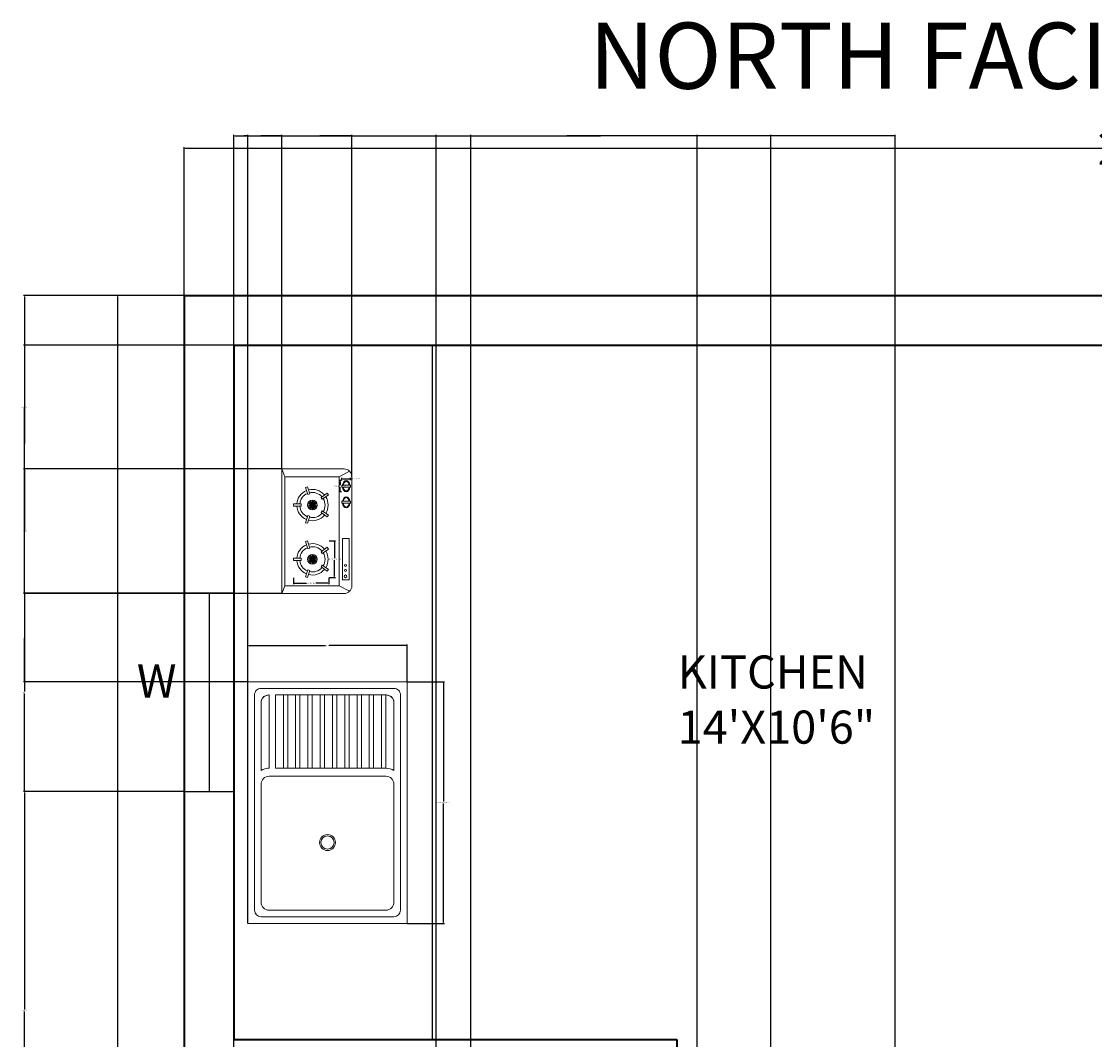
# Model space of a CAD drawing. Units: inches. Extents: x 3 to 420, y -502 to 54.
# Tile 5 of 6: x 3 to 198, y -130 to 54. Entities that reach past the tile are written whole.
import ezdxf

# ---------------------------------------------------------------- set-up
doc = ezdxf.new("R2010")
doc.units = ezdxf.units.IN
doc.header["$MEASUREMENT"] = 0
for name, color, linetype, lineweight in [('A-ANNO-DIMS', 2, 'Continuous', 18), ('A-ANNO-TEXT', 7, 'Continuous', 18), ('A-AREA-IDEN', 7, 'Continuous', 18), ('A-EQPM', 9, 'Continuous', 18), ('A-FLOR-CASE', 9, 'Continuous', 25), ('A-FLOR-FIXT', 9, 'Continuous', 18), ('A-GLAZ', 40, 'Continuous', 25), ('A-WALL', 7, 'Continuous', 35)]:
    doc.layers.add(name, color=color, linetype=linetype, lineweight=lineweight)
doc.styles.get("Standard").update_dxf_attribs({"font": 'arial.ttf'})
doc.dimstyles.get("Standard").update_dxf_attribs({"dimtxt": 0.18, "dimasz": 0.18, "dimexe": 0.18, "dimexo": 0.0625, "dimgap": 0.09, "dimtad": 0, "dimtih": 1, "dimtoh": 1, "dimdec": 0, "dimzin": 0, "dimdsep": 46, "dimlunit": 3, "dimtxsty": 'Standard', "dimcen": 0.09, "dimadec": 0, "dimazin": 0, "dimtfac": 1, "dimtdec": 0, "dimtofl": 0, "dimtmove": 0, "dimatfit": 3, "dimfxl": 1, "dimtolj": 1, "dimtzin": 0, "dimarcsym": 0})

# ---------------------------------------------------------------- blocks, each defined once
blk = doc.blocks.new('*D1')
at = {"layer": 'A-ANNO-DIMS', "color": 0, "lineweight": -2, "transparency": 16777216}
for p, q in [((32.39, 4.61), (32.39, 31.47)), ((32.57, 31.29), (198.86, 31.29)), ((390.71, 31.29), (224.42, 31.29)), ((390.89, 4.61), (390.89, 31.47))]:
    blk.add_line(p, q, dxfattribs=at)
at = {"layer": 'A-ANNO-DIMS', "color": 0, "transparency": 16777216}
for points in [[(32.57, 31.32), (32.57, 31.26), (32.39, 31.29)], [(390.71, 31.32), (390.71, 31.26), (390.89, 31.29)]]:
    blk.add_solid(points, dxfattribs=at)
at = {"layer": 'Defpoints', "color": 0, "transparency": 16777216}
for p in [(390.89, 31.29), (32.39, 4.54), (390.89, 4.54)]:
    blk.add_point(p, dxfattribs=at)
at = {"layer": 'A-ANNO-DIMS', "color": 0, "transparency": 16777216, "insert": (211.64, 31.29), "char_height": 6, "attachment_point": 5}
blk.add_mtext('\\A1;29\'-11"', dxfattribs=at)
blk = doc.blocks.new('*D2')
at = {"layer": 'A-ANNO-DIMS', "color": 0, "lineweight": -2, "transparency": 16777216}
for p, q in [((32.33, 4.54), (20.1, 4.54)), ((20.28, 4.36), (20.28, -230.8)), ((20.28, -472.28), (20.28, -237.11)), ((32.33, -472.46), (20.1, -472.46))]:
    blk.add_line(p, q, dxfattribs=at)
at = {"layer": 'A-ANNO-DIMS', "color": 0, "transparency": 16777216}
for points in [[(20.25, 4.36), (20.31, 4.36), (20.28, 4.54)], [(20.25, -472.28), (20.31, -472.28), (20.28, -472.46)]]:
    blk.add_solid(points, dxfattribs=at)
at = {"layer": 'Defpoints', "color": 0, "transparency": 16777216}
for p in [(32.39, 4.54), (20.28, -472.46), (32.39, -472.46)]:
    blk.add_point(p, dxfattribs=at)
at = {"layer": 'A-ANNO-DIMS', "color": 0, "transparency": 16777216, "insert": (20.28, -233.96), "char_height": 6, "attachment_point": 5}
blk.add_mtext('\\A1;39\'-9"', dxfattribs=at)
blk = doc.blocks.new('М12 540х820')
for p, q in [((0, 540), (-820, 540)), ((-820, 540), (-820, 0)), ((-45, 517.5), (-775, 517.5)), ((0, 0), (0, 540)), ((-797.5, 495), (-797.5, 45)), ((-347.5, 495), (-748, 495)), ((-301.7, 495), (-64.8, 495)), ((-22.5, 45), (-22.5, 495)), ((-775, 468), (-775, 72)), ((-320.5, 468), (-320.5, 72)), ((-293.7, 468), (-293.7, 472.5)), ((-293.7, 468), (-45, 468)), ((-293.7, 446.6), (-45, 446.6)), ((-293.7, 419.6), (-293.7, 446.6)), ((-45, 469.5), (-45, 468)), ((-45, 419.6), (-45, 446.6)), ((-293.7, 419.6), (-45, 419.6)), ((-293.7, 405), (-45, 405)), ((-293.7, 378), (-293.7, 405)), ((-45, 378), (-45, 405)), ((-293.7, 378), (-45, 378)), ((-293.7, 336.4), (-293.7, 363.4)), ((-293.7, 363.4), (-45, 363.4)), ((-293.7, 336.4), (-45, 336.4)), ((-45, 336.4), (-45, 363.4)), ((-293.7, 294.7), (-293.7, 321.7)), ((-293.7, 321.7), (-45, 321.7)), ((-293.7, 294.7), (-45, 294.7)), ((-45, 294.7), (-45, 321.7)), ((-293.7, 253.1), (-293.7, 280.1)), ((-293.7, 280.1), (-45, 280.1)), ((-45, 253.1), (-45, 280.1)), ((-293.7, 253.1), (-45, 253.1)), ((-293.7, 211.5), (-293.7, 238.5)), ((-293.7, 238.5), (-45, 238.5)), ((-45, 211.5), (-45, 238.5)), ((-293.7, 211.5), (-45, 211.5)), ((-293.7, 169.9), (-293.7, 196.9)), ((-293.7, 196.9), (-45, 196.9)), ((-45, 169.9), (-45, 196.9)), ((-293.7, 169.9), (-45, 169.9)), ((-293.7, 128.2), (-293.7, 155.2)), ((-293.7, 155.2), (-45, 155.2)), ((-45, 128.2), (-45, 155.2)), ((-293.7, 128.2), (-45, 128.2)), ((-293.7, 113.6), (-45, 113.6)), ((-293.7, 86.6), (-293.7, 113.6)), ((-45, 86.6), (-45, 113.6)), ((-293.7, 86.6), (-45, 86.6)), ((-748, 45), (-347.5, 45)), ((-301.7, 45), (-64.8, 45)), ((-293.7, 72), (-45, 72)), ((-45, 70.5), (-45, 72)), ((-820, 0), (0, 0)), ((-775, 22.5), (-45, 22.5))]:
    blk.add_line(p, q)
at = {"ltscale": 0.06}
for p, q in [((-820, 0), (-820, 540)), ((-820, 540), (0, 540)), ((0, 540), (0, 536.9)), ((0, 536.9), (0, 0)), ((-293.7, 446.6), (-45, 446.6)), ((-293.7, 405), (-293.7, 446.6)), ((-45, 446.6), (-45, 419.6)), ((-293.7, 363.4), (-293.7, 405)), ((-45, 419.6), (-45, 378)), ((-45, 378), (-45, 336.4)), ((-293.7, 321.7), (-293.7, 363.4)), ((-45, 336.4), (-45, 294.7)), ((-293.7, 280.1), (-293.7, 321.7)), ((-45, 294.7), (-45, 253.1)), ((-293.7, 238.5), (-293.7, 280.1)), ((-293.7, 196.9), (-293.7, 238.5)), ((-45, 253.1), (-45, 211.5)), ((-293.7, 155.2), (-293.7, 196.9)), ((-45, 211.5), (-45, 169.9)), ((-293.7, 113.6), (-293.7, 155.2)), ((-45, 169.9), (-45, 128.2)), ((-293.7, 72), (-293.7, 113.6)), ((-45, 128.2), (-45, 86.6)), ((-45, 86.6), (-45, 72)), ((-45, 72), (-293.7, 72)), ((0, 0), (-820, 0))]:
    blk.add_line(p, q, dxfattribs=at)
at = {"extrusion": (0, 0, -1)}
for centre, major_axis, start_param, end_param in [((-775, 495), (-15.9, 15.9), -0.785398, 0.785398), ((-775, 495), (-15.9, 15.9), -0.785398, 0.785398), ((-45, 495), (-15.9, -15.9), 2.356194, 3.926991), ((-45, 495), (-15.9, -15.9), 2.356194, 3.926991), ((-748, 468), (-19.1, -19.1), 0.785398, 2.356194), ((-748, 468), (-19.1, -19.1), 0.785398, 2.356194), ((-347.5, 468), (-19.1, 19.1), 0.785398, 2.356194), ((-347.5, 468), (-19.1, 19.1), 0.785398, 2.356194), ((-343.2, 468), (-35, 35), 1.779263, 2.356194), ((-343.2, 468), (-35, 35), 1.779263, 2.356192), ((-72.3, 468.8), (-19.3, 19.3), 1.0328, 2.38382), ((-72.3, 468.8), (-19.3, 19.3), 1.0328, 1.064673), ((-72.3, 468.8), (-19.3, 19.3), 1.064673, 2.328569), ((-343.2, 468), (-35, 35), 2.356192, 2.356194), ((-72.3, 468.8), (-19.3, 19.3), 2.328569, 2.38382), ((-545.5, 270), (-19.1, -19.1), 3.926991, 10.210176), ((-545.5, 270), (-19.1, -19.1), 3.926991, 10.210176), ((-545.5, 270), (-15.9, -15.9), 3.926991, 10.210176), ((-545.5, 270), (-15.9, -15.9), 3.926991, 10.210176), ((-775, 45), (-15.9, -15.9), 5.497787, 7.068583), ((-775, 45), (-15.9, -15.9), 5.497787, 7.068583), ((-748, 72), (-19.1, 19.1), 3.926991, 5.497787), ((-748, 72), (-19.1, 19.1), 3.926991, 5.497787), ((-347.5, 72), (-19.1, -19.1), 3.926991, 5.497787), ((-347.5, 72), (-19.1, -19.1), 3.926991, 5.497787), ((-343.2, 72), (-35, -35), 3.926991, 4.503922), ((-343.2, 72), (-35, -35), 3.926991, 4.503922), ((-72.3, 71.2), (-19.3, -19.3), 3.899365, 5.250385), ((-72.3, 71.2), (-19.3, -19.3), 5.218512, 5.250385), ((-72.3, 71.2), (-19.3, -19.3), 3.954617, 5.218512), ((-72.3, 71.2), (-19.3, -19.3), 3.899365, 3.954617), ((-45, 45), (-15.9, 15.9), 2.356194, 3.926991), ((-45, 45), (-15.9, 15.9), 2.356194, 3.926991)]:
    blk.add_ellipse(centre, major_axis=major_axis, ratio=1, start_param=start_param, end_param=end_param, dxfattribs=at)
blk = doc.blocks.new('COOKTOP-BURNER')
for p, q in [((2.19, 6.53), (2.56, 6.65)), ((2.61, 5.23), (2.19, 6.53)), ((2.56, 6.65), (2.98, 5.34)), ((2.98, 5.34), (2.61, 5.23)), ((3.43, 3.32), (2.92, 4.03)), ((3.43, 3.32), (3.16, 4.15)), ((3.43, 3.32), (3.43, 4.2)), ((3.43, 3.32), (3.7, 4.15)), ((3.43, 3.32), (3.95, 4.03)), ((4.99, 4.69), (6.1, 5.5)), ((5.21, 4.38), (4.99, 4.69)), ((6.32, 5.19), (5.21, 4.38)), ((6.1, 5.5), (6.32, 5.19)), ((0, 3.13), (0, 3.52)), ((0, 3.52), (1.37, 3.52)), ((1.37, 3.13), (0, 3.13)), ((1.37, 3.52), (1.37, 3.13)), ((3.43, 3.32), (2.56, 3.32)), ((3.43, 3.32), (2.61, 3.59)), ((3.43, 3.32), (2.61, 3.06)), ((3.43, 3.32), (2.73, 3.84)), ((3.43, 3.32), (2.73, 2.81)), ((3.43, 3.32), (2.92, 2.62)), ((3.43, 3.32), (3.16, 2.5)), ((3.43, 3.32), (4.14, 3.84)), ((3.43, 3.32), (4.26, 3.59)), ((3.43, 3.32), (3.43, 2.45)), ((3.43, 3.32), (3.7, 2.5)), ((3.43, 3.32), (3.95, 2.62)), ((3.43, 3.32), (4.14, 2.81)), ((3.43, 3.32), (4.26, 3.06)), ((3.43, 3.32), (4.3, 3.32)), ((4.99, 1.96), (5.21, 2.27)), ((6.1, 1.15), (4.99, 1.96)), ((5.21, 2.27), (6.32, 1.46)), ((2.19, 0.12), (2.61, 1.42)), ((2.56, 0), (2.19, 0.12)), ((2.98, 1.31), (2.56, 0)), ((2.61, 1.42), (2.98, 1.31)), ((6.32, 1.46), (6.1, 1.15))]:
    blk.add_line(p, q)
blk.add_circle((3.43, 3.32), 0.875)
for radius, start, end in [(2.85, 111.8765, 176.1235), (2.85, 39.8765, 104.1235), (2.29, 112.8365, 175.1635), (2.29, 40.8365, 103.1635), (2.29, 328.8365, 31.1635), (2.85, 327.8765, 32.1235), (2.85, 183.8765, 248.1235), (2.29, 184.8365, 247.1635), (2.85, 255.8765, 320.1235), (2.29, 256.8365, 319.1635)]:
    blk.add_arc((3.43, 3.32), radius, start, end)
blk = doc.blocks.new('COOKTOP-CONTROL')
for p, q in [((0, 0.85), (0, 1.22)), ((0, 1.22), (1.56, 1.22)), ((1.56, 0.85), (0, 0.85)), ((1.56, 1.22), (1.56, 0.85))]:
    blk.add_line(p, q)
for major_axis, start_param, end_param in [((0, -1.01), 1.774361, 4.508825), ((0, 1.01), 1.73081, 4.552375)]:
    blk.add_ellipse((0.79, 1.01), major_axis=major_axis, ratio=0.671641, start_param=start_param, end_param=end_param)
for points, knots in [([(0.26, 0.85), (0.27, 0.81), (0.27, 0.78), (0.29, 0.68), (0.31, 0.62), (0.35, 0.5), (0.38, 0.45), (0.44, 0.36), (0.47, 0.32), (0.53, 0.25), (0.57, 0.22), (0.64, 0.18), (0.67, 0.16), (0.73, 0.14), (0.76, 0.14), (0.79, 0.14), (0.82, 0.14), (0.86, 0.15), (0.93, 0.17), (0.96, 0.19), (1.03, 0.23), (1.06, 0.26), (1.13, 0.34), (1.16, 0.38), (1.21, 0.48), (1.24, 0.53), (1.28, 0.65), (1.29, 0.71), (1.31, 0.8), (1.31, 0.82), (1.32, 0.85)], [4.889299, 4.889299, 4.889299, 4.889299, 5.015191, 5.015191, 5.233243, 5.233243, 5.451295, 5.451295, 5.669347, 5.669347, 5.887399, 5.887399, 6.10545, 6.10545, 6.283185, 6.283185, 6.283185, 6.501237, 6.501237, 6.719289, 6.719289, 6.937341, 6.937341, 7.155392, 7.155392, 7.373444, 7.373444, 7.591496, 7.591496, 7.677072, 7.677072, 7.677072, 7.677072]), ([(1.31, 1.22), (1.3, 1.27), (1.29, 1.31), (1.26, 1.42), (1.24, 1.48), (1.19, 1.58), (1.17, 1.63), (1.1, 1.72), (1.07, 1.75), (1, 1.81), (0.97, 1.83), (0.9, 1.86), (0.87, 1.87), (0.8, 1.88), (0.76, 1.88), (0.69, 1.87), (0.66, 1.86), (0.59, 1.82), (0.56, 1.79), (0.49, 1.73), (0.46, 1.69), (0.4, 1.61), (0.37, 1.56), (0.32, 1.45), (0.3, 1.39), (0.28, 1.29), (0.27, 1.25), (0.27, 1.22)], [8.079302, 8.079302, 8.079302, 8.079302, 8.245651, 8.245651, 8.463703, 8.463703, 8.681755, 8.681755, 8.899807, 8.899807, 9.117859, 9.117859, 9.33591, 9.33591, 9.553962, 9.553962, 9.772014, 9.772014, 9.990066, 9.990066, 10.208118, 10.208118, 10.426169, 10.426169, 10.644221, 10.644221, 10.770253, 10.770253, 10.770253, 10.770253])]:
    blk.add_open_spline(points, degree=3, knots=knots)
blk = doc.blocks.new('*D33')
at = {"layer": 'A-ANNO-DIMS', "color": 0, "lineweight": -2, "transparency": 16777216}
for p, q in [((58.7, -39.98), (59.82, -39.98)), ((59.64, -40.16), (59.64, -43.12)), ((59.64, -46.45), (59.64, -43.49)), ((58.7, -46.63), (59.82, -46.63))]:
    blk.add_line(p, q, dxfattribs=at)
at = {"layer": 'A-ANNO-DIMS', "color": 0, "transparency": 16777216}
for points in [[(59.61, -40.16), (59.67, -40.16), (59.64, -39.98)], [(59.61, -46.45), (59.67, -46.45), (59.64, -46.63)]]:
    blk.add_solid(points, dxfattribs=at)
at = {"layer": 'Defpoints', "color": 0, "transparency": 16777216}
for p in [(58.64, -39.98), (59.64, -39.98), (58.64, -46.63)]:
    blk.add_point(p, dxfattribs=at)
at = {"layer": 'A-ANNO-DIMS', "color": 0, "transparency": 16777216, "insert": (59.64, -43.31), "char_height": 0.18, "attachment_point": 5}
blk.add_mtext('\\A1;BURNER 0\'-6 1/2" TYP.', dxfattribs=at)
blk = doc.blocks.new('*D34')
at = {"layer": 'A-ANNO-DIMS', "color": 0, "lineweight": -2, "transparency": 16777216}
for p, q in [((52.21, -46.69), (52.21, -47.81)), ((58.64, -46.69), (58.64, -47.81)), ((52.39, -47.63), (54.58, -47.63)), ((58.46, -47.63), (56.27, -47.63))]:
    blk.add_line(p, q, dxfattribs=at)
at = {"layer": 'A-ANNO-DIMS', "color": 0, "transparency": 16777216}
for points in [[(52.39, -47.6), (52.39, -47.66), (52.21, -47.63)], [(58.46, -47.6), (58.46, -47.66), (58.64, -47.63)]]:
    blk.add_solid(points, dxfattribs=at)
at = {"layer": 'Defpoints', "color": 0, "transparency": 16777216}
for p in [(52.21, -46.63), (58.64, -46.63), (58.64, -47.63)]:
    blk.add_point(p, dxfattribs=at)
at = {"layer": 'A-ANNO-DIMS', "color": 0, "transparency": 16777216, "insert": (55.43, -47.63), "char_height": 0.18, "attachment_point": 5}
blk.add_mtext('\\A1;0\'-6 1/2" TYP.', dxfattribs=at)
blk = doc.blocks.new('*D35')
at = {"layer": 'A-ANNO-DIMS', "color": 0, "lineweight": -2, "transparency": 16777216}
for p, q in [((60.92, -29.03), (60.49, -29.03)), ((60.92, -31.05), (60.49, -31.05)), ((60.67, -29.21), (60.67, -29.85)), ((60.67, -30.87), (60.67, -30.22))]:
    blk.add_line(p, q, dxfattribs=at)
at = {"layer": 'A-ANNO-DIMS', "color": 0, "transparency": 16777216}
for points in [[(60.64, -29.21), (60.7, -29.21), (60.67, -29.03)], [(60.64, -30.87), (60.7, -30.87), (60.67, -31.05)]]:
    blk.add_solid(points, dxfattribs=at)
at = {"layer": 'Defpoints', "color": 0, "transparency": 16777216}
for p in [(60.67, -29.03), (60.98, -29.03), (60.98, -31.05)]:
    blk.add_point(p, dxfattribs=at)
at = {"layer": 'A-ANNO-DIMS', "color": 0, "transparency": 16777216, "insert": (60.67, -30.04), "char_height": 0.18, "attachment_point": 5}
blk.add_mtext('\\A1;CONTROL 0\'-2" TYP.', dxfattribs=at)
blk = doc.blocks.new('*D36')
at = {"layer": 'A-ANNO-DIMS', "color": 0, "lineweight": -2, "transparency": 16777216}
for p, q in [((60.98, -28.96), (60.98, -28.54)), ((61.16, -28.72), (62.36, -28.72)), ((62.54, -28.96), (62.54, -28.54)), ((62.54, -28.72), (62.72, -28.72))]:
    blk.add_line(p, q, dxfattribs=at)
at = {"layer": 'A-ANNO-DIMS', "color": 0, "transparency": 16777216}
for points in [[(61.16, -28.69), (61.16, -28.75), (60.98, -28.72)], [(62.36, -28.69), (62.36, -28.75), (62.54, -28.72)]]:
    blk.add_solid(points, dxfattribs=at)
at = {"layer": 'Defpoints', "color": 0, "transparency": 16777216}
for p in [(60.98, -29.03), (62.54, -28.72), (62.54, -29.03)]:
    blk.add_point(p, dxfattribs=at)
at = {"layer": 'A-ANNO-DIMS', "color": 0, "transparency": 16777216, "insert": (63.57, -28.72), "char_height": 0.18, "attachment_point": 5}
blk.add_mtext('\\A1;0\'-1 1/2" TYP.', dxfattribs=at)
blk = doc.blocks.new('*D37')
at = {"layer": 'A-ANNO-DIMS', "color": 0, "lineweight": -2, "transparency": 16777216}
for p, q in [((72.88, -65.52), (79.58, -65.52)), ((79.4, -65.7), (79.4, -87.27)), ((79.4, -109.21), (79.4, -87.64)), ((72.88, -109.39), (79.58, -109.39))]:
    blk.add_line(p, q, dxfattribs=at)
at = {"layer": 'A-ANNO-DIMS', "color": 0, "transparency": 16777216}
for points in [[(79.37, -65.7), (79.43, -65.7), (79.4, -65.52)], [(79.37, -109.21), (79.43, -109.21), (79.4, -109.39)]]:
    blk.add_solid(points, dxfattribs=at)
at = {"layer": 'Defpoints', "color": 0, "transparency": 16777216}
for p in [(72.82, -65.52), (79.4, -65.52), (72.82, -109.39)]:
    blk.add_point(p, dxfattribs=at)
at = {"layer": 'A-ANNO-DIMS', "color": 0, "transparency": 16777216, "insert": (79.4, -87.45), "char_height": 0.18, "attachment_point": 5}
blk.add_mtext('\\A1;SINK & DRAINER 3\'-8"', dxfattribs=at)
blk = doc.blocks.new('*D38')
at = {"layer": 'A-ANNO-DIMS', "color": 0, "lineweight": -2, "transparency": 16777216}
for p, q in [((43.93, -65.45), (43.93, -58.76)), ((44.11, -58.94), (58.04, -58.94)), ((72.64, -58.94), (58.7, -58.94)), ((72.82, -65.45), (72.82, -58.76))]:
    blk.add_line(p, q, dxfattribs=at)
at = {"layer": 'A-ANNO-DIMS', "color": 0, "transparency": 16777216}
for points in [[(44.11, -58.91), (44.11, -58.97), (43.93, -58.94)], [(72.64, -58.91), (72.64, -58.97), (72.82, -58.94)]]:
    blk.add_solid(points, dxfattribs=at)
at = {"layer": 'Defpoints', "color": 0, "transparency": 16777216}
for p in [(43.93, -58.94), (43.93, -65.52), (72.82, -65.52)]:
    blk.add_point(p, dxfattribs=at)
at = {"layer": 'A-ANNO-DIMS', "color": 0, "transparency": 16777216, "insert": (58.37, -58.94), "char_height": 0.18, "attachment_point": 5}
blk.add_mtext('\\A1;2\'-5"', dxfattribs=at)
blk = doc.blocks.new('*D40')
at = {"layer": 'A-ANNO-DIMS', "color": 0, "lineweight": -2, "transparency": 16777216}
for p, q in [((50.07, -26.84), (50.07, 33.72)), ((50.25, 33.54), (55.9, 33.54)), ((62.62, 33.54), (56.97, 33.54)), ((62.8, -28.26), (62.8, 33.72))]:
    blk.add_line(p, q, dxfattribs=at)
at = {"layer": 'A-ANNO-DIMS', "color": 0, "transparency": 16777216}
for points in [[(50.25, 33.57), (50.25, 33.51), (50.07, 33.54)], [(62.62, 33.57), (62.62, 33.51), (62.8, 33.54)]]:
    blk.add_solid(points, dxfattribs=at)
at = {"layer": 'Defpoints', "color": 0, "transparency": 16777216}
for p in [(62.8, 33.54), (50.07, -26.9), (62.8, -28.32)]:
    blk.add_point(p, dxfattribs=at)
at = {"layer": 'A-ANNO-DIMS', "color": 0, "transparency": 16777216, "insert": (56.44, 33.54), "char_height": 0.18, "attachment_point": 5}
blk.add_mtext('\\A1;1\'-0 1/2"', dxfattribs=at)
blk = doc.blocks.new('*D41')
at = {"layer": 'A-ANNO-DIMS', "color": 0, "lineweight": -2, "transparency": 16777216}
for p, q in [((50.01, -26.9), (3.21, -26.9)), ((3.39, -27.08), (3.39, -38.03)), ((3.39, -49.34), (3.39, -38.4)), ((50.01, -49.52), (3.21, -49.52))]:
    blk.add_line(p, q, dxfattribs=at)
at = {"layer": 'A-ANNO-DIMS', "color": 0, "transparency": 16777216}
for points in [[(3.36, -27.08), (3.42, -27.08), (3.39, -26.9)], [(3.36, -49.34), (3.42, -49.34), (3.39, -49.52)]]:
    blk.add_solid(points, dxfattribs=at)
at = {"layer": 'Defpoints', "color": 0, "transparency": 16777216}
for p in [(50.07, -26.9), (3.39, -49.52), (50.07, -49.52)]:
    blk.add_point(p, dxfattribs=at)
at = {"layer": 'A-ANNO-DIMS', "color": 0, "transparency": 16777216, "insert": (3.39, -38.21), "char_height": 0.18, "attachment_point": 5}
blk.add_mtext('\\A1;1\'-10 1/2"', dxfattribs=at)
blk = doc.blocks.new('*D42')
at = {"layer": 'A-ANNO-DIMS', "color": 0, "lineweight": -2, "transparency": 16777216}
for p, q in [((50.01, -49.52), (3.21, -49.52)), ((3.39, -49.7), (3.39, -57.34)), ((3.39, -65.34), (3.39, -57.7)), ((43.86, -65.52), (3.21, -65.52))]:
    blk.add_line(p, q, dxfattribs=at)
at = {"layer": 'A-ANNO-DIMS', "color": 0, "transparency": 16777216}
for points in [[(3.36, -49.7), (3.42, -49.7), (3.39, -49.52)], [(3.36, -65.34), (3.42, -65.34), (3.39, -65.52)]]:
    blk.add_solid(points, dxfattribs=at)
at = {"layer": 'Defpoints', "color": 0, "transparency": 16777216}
for p in [(50.07, -49.52), (3.39, -65.52), (43.93, -65.52)]:
    blk.add_point(p, dxfattribs=at)
at = {"layer": 'A-ANNO-DIMS', "color": 0, "transparency": 16777216, "insert": (3.39, -57.52), "char_height": 0.18, "attachment_point": 5}
blk.add_mtext('\\A1;1\'-4"', dxfattribs=at)
blk = doc.blocks.new('*D43')
at = {"layer": 'A-ANNO-DIMS', "color": 0, "lineweight": -2, "transparency": 16777216}
for p, q in [((41.33, -4.46), (3.21, -4.46)), ((3.39, -4.64), (3.39, -15.5)), ((3.39, -26.72), (3.39, -15.86)), ((50.01, -26.9), (3.21, -26.9))]:
    blk.add_line(p, q, dxfattribs=at)
at = {"layer": 'A-ANNO-DIMS', "color": 0, "transparency": 16777216}
for points in [[(3.36, -4.64), (3.42, -4.64), (3.39, -4.46)], [(3.36, -26.72), (3.42, -26.72), (3.39, -26.9)]]:
    blk.add_solid(points, dxfattribs=at)
at = {"layer": 'Defpoints', "color": 0, "transparency": 16777216}
for p in [(3.39, -4.46), (41.39, -4.46), (50.07, -26.9)]:
    blk.add_point(p, dxfattribs=at)
at = {"layer": 'A-ANNO-DIMS', "color": 0, "transparency": 16777216, "insert": (3.39, -15.68), "char_height": 0.18, "attachment_point": 5}
blk.add_mtext('\\A1;1\'-10 1/2"', dxfattribs=at)
blk = doc.blocks.new('*D44')
at = {"layer": 'A-ANNO-DIMS', "color": 0, "lineweight": -2, "transparency": 16777216}
for p, q in [((41.39, -4.39), (41.39, 33.72)), ((41.57, 33.54), (45.19, 33.54)), ((49.89, 33.54), (46.27, 33.54)), ((50.07, -26.84), (50.07, 33.72))]:
    blk.add_line(p, q, dxfattribs=at)
at = {"layer": 'A-ANNO-DIMS', "color": 0, "transparency": 16777216}
for points in [[(41.57, 33.57), (41.57, 33.51), (41.39, 33.54)], [(49.89, 33.57), (49.89, 33.51), (50.07, 33.54)]]:
    blk.add_solid(points, dxfattribs=at)
at = {"layer": 'Defpoints', "color": 0, "transparency": 16777216}
for p in [(50.07, 33.54), (41.39, -4.46), (50.07, -26.9)]:
    blk.add_point(p, dxfattribs=at)
at = {"layer": 'A-ANNO-DIMS', "color": 0, "transparency": 16777216, "insert": (45.73, 33.54), "char_height": 0.18, "attachment_point": 5}
blk.add_mtext('\\A1;0\'-8 1/2"', dxfattribs=at)
blk = doc.blocks.new('*D45')
at = {"layer": 'A-ANNO-DIMS', "color": 0, "lineweight": -2, "transparency": 16777216}
for p, q in [((41.39, -130.39), (41.39, 33.72)), ((41.57, 33.54), (42.12, 33.54)), ((43.75, 33.54), (43.2, 33.54)), ((43.93, -109.33), (43.93, 33.72))]:
    blk.add_line(p, q, dxfattribs=at)
at = {"layer": 'A-ANNO-DIMS', "color": 0, "transparency": 16777216}
for points in [[(41.57, 33.57), (41.57, 33.51), (41.39, 33.54)], [(43.75, 33.57), (43.75, 33.51), (43.93, 33.54)]]:
    blk.add_solid(points, dxfattribs=at)
at = {"layer": 'Defpoints', "color": 0, "transparency": 16777216}
for p in [(41.39, 33.54), (43.93, -109.39), (41.39, -130.46)]:
    blk.add_point(p, dxfattribs=at)
at = {"layer": 'A-ANNO-DIMS', "color": 0, "transparency": 16777216, "insert": (42.66, 33.54), "char_height": 0.18, "attachment_point": 5}
blk.add_mtext('\\A1;0\'-2 1/2"', dxfattribs=at)
blk = doc.blocks.new('*D47')
at = {"layer": 'A-ANNO-DIMS', "color": 0, "lineweight": -2, "transparency": 16777216}
for p, q in [((41.39, -254.89), (41.39, 33.72)), ((41.57, 33.54), (101, 33.54)), ((161.2, 33.54), (101.78, 33.54)), ((161.38, -254.89), (161.38, 33.72))]:
    blk.add_line(p, q, dxfattribs=at)
at = {"layer": 'A-ANNO-DIMS', "color": 0, "transparency": 16777216}
for points in [[(41.57, 33.57), (41.57, 33.51), (41.39, 33.54)], [(161.2, 33.57), (161.2, 33.51), (161.38, 33.54)]]:
    blk.add_solid(points, dxfattribs=at)
at = {"layer": 'Defpoints', "color": 0, "transparency": 16777216}
for p in [(161.38, 33.54), (41.39, -254.96), (161.38, -254.96)]:
    blk.add_point(p, dxfattribs=at)
at = {"layer": 'A-ANNO-DIMS', "color": 0, "transparency": 16777216, "insert": (101.39, 33.54), "char_height": 0.18, "attachment_point": 5}
blk.add_mtext('\\A1;10\'-0"', dxfattribs=at)
blk = doc.blocks.new('*D48')
at = {"layer": 'A-ANNO-DIMS', "color": 0, "lineweight": -2, "transparency": 16777216}
for p, q in [((32.33, -49.46), (3.21, -49.46)), ((3.39, -49.64), (3.39, -67.27)), ((3.39, -85.28), (3.39, -67.64)), ((32.33, -85.46), (3.21, -85.46))]:
    blk.add_line(p, q, dxfattribs=at)
at = {"layer": 'A-ANNO-DIMS', "color": 0, "transparency": 16777216}
for points in [[(3.36, -49.64), (3.42, -49.64), (3.39, -49.46)], [(3.36, -85.28), (3.42, -85.28), (3.39, -85.46)]]:
    blk.add_solid(points, dxfattribs=at)
at = {"layer": 'Defpoints', "color": 0, "transparency": 16777216}
for p in [(32.39, -49.46), (3.39, -85.46), (32.39, -85.46)]:
    blk.add_point(p, dxfattribs=at)
at = {"layer": 'A-ANNO-DIMS', "color": 0, "transparency": 16777216, "insert": (3.39, -67.46), "char_height": 0.18, "attachment_point": 5}
blk.add_mtext('\\A1;3\'-0"', dxfattribs=at)
blk = doc.blocks.new('*D59')
at = {"layer": 'A-ANNO-DIMS', "color": 0, "lineweight": -2, "transparency": 16777216}
for p, q in [((32.33, 4.54), (3.21, 4.54)), ((3.39, 4.36), (3.39, -22.27)), ((3.39, -49.28), (3.39, -22.64)), ((32.33, -49.46), (3.21, -49.46))]:
    blk.add_line(p, q, dxfattribs=at)
at = {"layer": 'A-ANNO-DIMS', "color": 0, "transparency": 16777216}
for points in [[(3.36, 4.36), (3.42, 4.36), (3.39, 4.54)], [(3.36, -49.28), (3.42, -49.28), (3.39, -49.46)]]:
    blk.add_solid(points, dxfattribs=at)
at = {"layer": 'Defpoints', "color": 0, "transparency": 16777216}
for p in [(32.39, 4.54), (3.39, -49.46), (32.39, -49.46)]:
    blk.add_point(p, dxfattribs=at)
at = {"layer": 'A-ANNO-DIMS', "color": 0, "transparency": 16777216, "insert": (3.39, -22.46), "char_height": 0.18, "attachment_point": 5}
blk.add_mtext('\\A1;4\'-6"', dxfattribs=at)
blk = doc.blocks.new('*D60')
at = {"layer": 'A-ANNO-DIMS', "color": 0, "lineweight": -2, "transparency": 16777216}
for p, q in [((32.33, -85.46), (3.21, -85.46)), ((3.39, -85.64), (3.39, -125.02)), ((3.39, -164.78), (3.39, -125.39)), ((32.33, -164.96), (3.21, -164.96))]:
    blk.add_line(p, q, dxfattribs=at)
at = {"layer": 'A-ANNO-DIMS', "color": 0, "transparency": 16777216}
for points in [[(3.36, -85.64), (3.42, -85.64), (3.39, -85.46)], [(3.36, -164.78), (3.42, -164.78), (3.39, -164.96)]]:
    blk.add_solid(points, dxfattribs=at)
at = {"layer": 'Defpoints', "color": 0, "transparency": 16777216}
for p in [(32.39, -85.46), (3.39, -164.96), (32.39, -164.96)]:
    blk.add_point(p, dxfattribs=at)
at = {"layer": 'A-ANNO-DIMS', "color": 0, "transparency": 16777216, "insert": (3.39, -125.21), "char_height": 0.18, "attachment_point": 5}
blk.add_mtext('\\A1;6\'-7 1/2"', dxfattribs=at)
blk = doc.blocks.new('*D62')
at = {"layer": 'A-ANNO-DIMS', "color": 0, "lineweight": -2, "transparency": 16777216}
for p, q in [((84.39, -463.39), (84.39, 33.72)), ((84.57, 33.54), (104.58, 33.54)), ((125.25, 33.54), (105.24, 33.54)), ((125.43, -463.39), (125.43, 33.72))]:
    blk.add_line(p, q, dxfattribs=at)
at = {"layer": 'A-ANNO-DIMS', "color": 0, "transparency": 16777216}
for points in [[(84.57, 33.57), (84.57, 33.51), (84.39, 33.54)], [(125.25, 33.57), (125.25, 33.51), (125.43, 33.54)]]:
    blk.add_solid(points, dxfattribs=at)
at = {"layer": 'Defpoints', "color": 0, "transparency": 16777216}
for p in [(125.43, 33.54), (84.39, -463.46), (125.43, -463.46)]:
    blk.add_point(p, dxfattribs=at)
at = {"layer": 'A-ANNO-DIMS', "color": 0, "transparency": 16777216, "insert": (104.91, 33.54), "char_height": 0.18, "attachment_point": 5}
blk.add_mtext('\\A1;3\'-5"', dxfattribs=at)
blk = doc.blocks.new('*D71')
at = {"layer": 'A-ANNO-DIMS', "color": 0, "lineweight": -2, "transparency": 16777216}
for p, q in [((78.09, -174.49), (78.09, 33.72)), ((78.27, 33.54), (107.89, 33.54)), ((138.59, 33.54), (108.97, 33.54)), ((138.77, -174.49), (138.77, 33.72))]:
    blk.add_line(p, q, dxfattribs=at)
at = {"layer": 'A-ANNO-DIMS', "color": 0, "transparency": 16777216}
for points in [[(78.27, 33.57), (78.27, 33.51), (78.09, 33.54)], [(138.59, 33.57), (138.59, 33.51), (138.77, 33.54)]]:
    blk.add_solid(points, dxfattribs=at)
at = {"layer": 'Defpoints', "color": 0, "transparency": 16777216}
for p in [(138.77, 33.54), (78.09, -174.56), (138.77, -174.56)]:
    blk.add_point(p, dxfattribs=at)
at = {"layer": 'A-ANNO-DIMS', "color": 0, "transparency": 16777216, "insert": (108.43, 33.54), "char_height": 0.18, "attachment_point": 5}
blk.add_mtext('\\A1;5\'-0 1/2"', dxfattribs=at)

msp = doc.modelspace()

# ---------------------------------------------------------------- linework, layer by layer
at = {"layer": 'A-EQPM'}
for p, q in [((61.38, -26.9), (50.07, -26.9)), ((50.07, -26.9), (50.07, -49.52)), ((50.61, -28.32), (50.07, -26.9)), ((60.51, -28.32), (50.61, -28.32)), ((50.61, -28.32), (50.61, -48.11)), ((60.51, -28.32), (62.38, -27.32)), ((60.51, -48.11), (60.51, -28.32)), ((62.8, -48.11), (62.8, -28.32)), ((61.1, -47.03), (61.1, -39.54)), ((61.1, -39.54), (62.31, -39.54)), ((62.31, -39.54), (62.31, -47.03)), ((50.61, -48.11), (50.07, -49.52)), ((50.61, -48.11), (60.51, -48.11)), ((60.51, -48.11), (62.38, -49.11)), ((62.31, -47.03), (61.1, -47.03)), ((50.07, -49.52), (61.38, -49.52))]:
    msp.add_line(p, q, dxfattribs=at)
for centre, radius in [((61.64, -44.39), 0.209), ((61.64, -46.4), 0.251), ((61.64, -45.31), 0.209)]:
    msp.add_circle(centre, radius, dxfattribs=at)
for centre, start, end in [((61.38, -28.32), 0, 90), ((61.38, -48.11), 270, 0)]:
    msp.add_arc(centre, 1.41, start, end, dxfattribs=at)
at = {"layer": 'A-FLOR-CASE'}
msp.add_line((77.36, -4.46), (77.36, -130.46), dxfattribs=at)
at = {"layer": 'A-GLAZ'}
for p, q in [((32.39, -49.46), (32.39, -85.46)), ((41.39, -49.46), (32.39, -49.46)), ((36.89, -49.46), (36.89, -85.46)), ((41.39, -85.46), (41.39, -49.46)), ((32.39, -85.46), (41.39, -85.46))]:
    msp.add_line(p, q, dxfattribs=at)
at = {"layer": 'A-WALL'}
for p, q in [((32.39, 4.54), (32.39, -472.46)), ((32.39, 4.54), (390.89, 4.54)), ((41.39, -4.46), (41.39, -130.46)), ((41.39, -4.46), (209.39, -4.46)), ((41.39, -130.46), (121.75, -130.46)), ((121.75, -130.46), (121.75, -134.96))]:
    msp.add_line(p, q, dxfattribs=at)

# ---------------------------------------------------------------- block references
at = {"layer": 'A-EQPM'}
for name, p in [('COOKTOP-CONTROL', (60.98, -31.05)), ('COOKTOP-BURNER', (52.21, -36.78)), ('COOKTOP-CONTROL', (60.98, -33.98)), ('COOKTOP-BURNER', (52.21, -46.63))]:
    msp.add_blockref(name, p, dxfattribs=at)
at = {"layer": 'A-FLOR-FIXT', "xscale": 0.0535008168779169, "yscale": 0.0535008168779169, "zscale": 0.0535008168779169, "rotation": 90}
msp.add_blockref('М12 540х820', (72.82, -65.52), dxfattribs=at)

# ---------------------------------------------------------------- texts
at = {"layer": 'A-ANNO-TEXT', "attachment_point": 1}
for s, insert, char_height in [('NORTH FACING HOUSE', (105.86, 54.08), 12), ('W', (23.79, -62.39), 6)]:
    msp.add_mtext(s, dxfattribs=dict(at, insert=insert, char_height=char_height))
at = {"layer": 'A-AREA-IDEN', "insert": (121.89, -60.76), "char_height": 6, "attachment_point": 1}
msp.add_mtext('KITCHEN\\P14\'X10\'6"', dxfattribs=at)

# ---------------------------------------------------------------- dimensions: what is measured, and where the dimension line sits
at = {"layer": 'A-ANNO-DIMS'}
for base, p1, p2, override, picture, middle in [((390.88918496, 31.29388447), (32.38918496, 4.54371834), (390.88918496, 4.54371834), {"dimtxt": 6, "dimclrd": 0, "dimclre": 0, "dimclrt": 0}, '*D1', (211.63918496, 31.29388447)), ((50.07, 33.54), (41.39, -4.46), (50.07, -26.9), {"dimdec": 1, "dimlfac": 1, "dimrnd": 0, "dimzin": 1, "dimdsep": 46, "dimlunit": 4, "dimfrac": 2}, '*D44', (45.73, 33.54)), ((41.39, 33.54), (43.93, -109.39), (41.39, -130.46), {"dimdec": 1, "dimlfac": 1, "dimrnd": 0, "dimzin": 1, "dimdsep": 46, "dimlunit": 4, "dimfrac": 2}, '*D45', (42.66, 33.54)), ((161.38, 33.54), (41.39, -254.96), (161.38, -254.96), {"dimdec": 1, "dimlfac": 1, "dimrnd": 0, "dimzin": 1, "dimdsep": 46, "dimlunit": 4, "dimfrac": 2}, '*D47', (101.39, 33.54)), ((62.8, 33.54), (50.07, -26.9), (62.8, -28.32), {"dimdec": 1, "dimlfac": 1, "dimrnd": 0, "dimzin": 1, "dimdsep": 46, "dimlunit": 4, "dimfrac": 2}, '*D40', (56.44, 33.54)), ((138.77, 33.54), (78.09, -174.56), (138.77, -174.56), {"dimdec": 1, "dimlfac": 1, "dimrnd": 0, "dimzin": 1, "dimdsep": 46, "dimlunit": 4, "dimfrac": 2}, '*D71', (108.43, 33.54)), ((125.43, 33.54), (84.39, -463.46), (125.43, -463.46), {"dimdec": 1, "dimlfac": 1, "dimrnd": 0, "dimzin": 1, "dimdsep": 46, "dimlunit": 4, "dimfrac": 2}, '*D62', (104.91, 33.54))]:
    dim = msp.add_linear_dim(base=base, p1=p1, p2=p2, dimstyle='Standard', override=override, dxfattribs=at)
    dim.commit()
    dim.dimension.update_dxf_attribs({"geometry": picture, "text_midpoint": middle})
for base, p1, p2, angle, override, picture, middle in [((3.39, -49.46), (32.39, 4.54), (32.39, -49.46), 90, {"dimdec": 1, "dimlfac": 1, "dimrnd": 0, "dimzin": 1, "dimdsep": 46, "dimlunit": 4, "dimfrac": 2}, '*D59', (3.39, -22.46)), ((20.28, -472.46), (32.39, 4.54), (32.39, -472.46), 90, {"dimtxt": 6, "dimclrd": 0, "dimclre": 0, "dimclrt": 0}, '*D2', (20.28, -233.96)), ((3.39, -4.46), (50.07, -26.9), (41.39, -4.46), 90, {"dimdec": 1, "dimlfac": 1, "dimrnd": 0, "dimzin": 1, "dimdsep": 46, "dimlunit": 4, "dimfrac": 2}, '*D43', (3.39, -15.68)), ((3.39, -49.52), (50.07, -26.9), (50.07, -49.52), 90, {"dimdec": 1, "dimlfac": 1, "dimrnd": 0, "dimzin": 1, "dimdsep": 46, "dimlunit": 4, "dimfrac": 2}, '*D41', (3.39, -38.21)), ((3.39, -85.46), (32.39, -49.46), (32.39, -85.46), 90, {"dimdec": 1, "dimlfac": 1, "dimrnd": 0, "dimzin": 1, "dimdsep": 46, "dimlunit": 4, "dimfrac": 2}, '*D48', (3.39, -67.46)), ((3.39, -65.52), (50.07, -49.52), (43.93, -65.52), 90, {"dimdec": 1, "dimlfac": 1, "dimrnd": 0, "dimzin": 1, "dimdsep": 46, "dimlunit": 4, "dimfrac": 2}, '*D42', (3.39, -57.52)), ((43.93, -58.94), (72.82, -65.52), (43.93, -65.52), 180, {"dimdec": 1, "dimlfac": 1, "dimrnd": 0, "dimzin": 1, "dimdsep": 46, "dimlunit": 4, "dimfrac": 2}, '*D38', (58.37, -58.94)), ((3.39, -164.96), (32.39, -85.46), (32.39, -164.96), 90, {"dimdec": 1, "dimlfac": 1, "dimrnd": 0, "dimzin": 1, "dimdsep": 46, "dimlunit": 4, "dimfrac": 2}, '*D60', (3.39, -125.21))]:
    dim = msp.add_linear_dim(base=base, p1=p1, p2=p2, angle=angle, dimstyle='Standard', override=override, dxfattribs=at)
    dim.commit()
    dim.dimension.update_dxf_attribs({"geometry": picture, "text_midpoint": middle})
for base, p1, p2, text, picture, middle in [((60.67, -29.03), (60.98, -31.05), (60.98, -29.03), 'CONTROL <> TYP.', '*D35', (60.67, -30.04)), ((59.6392, -39.9801), (58.6417, -46.6302), (58.6417, -39.9801), 'BURNER <> TYP.', '*D33', (59.6392, -43.3051)), ((79.4, -65.52), (72.82, -109.39), (72.82, -65.52), 'SINK & DRAINER <>', '*D37', (79.4, -87.45))]:
    dim = msp.add_linear_dim(base=base, p1=p1, p2=p2, angle=90, text=text, dimstyle='Standard', override={"dimdec": 1, "dimlfac": 1, "dimrnd": 0, "dimzin": 1, "dimdsep": 46, "dimlunit": 4, "dimfrac": 2}, dxfattribs=at)
    dim.commit()
    dim.dimension.update_dxf_attribs({"geometry": picture, "text_midpoint": middle})
for base, p1, p2, picture, middle in [((62.54, -28.72), (60.98, -29.03), (62.54, -29.03), '*D36', (63.57, -28.72)), ((58.64, -47.63), (52.21, -46.63), (58.64, -46.63), '*D34', (55.43, -47.63))]:
    dim = msp.add_linear_dim(base=base, p1=p1, p2=p2, text='<> TYP.', dimstyle='Standard', override={"dimdec": 1, "dimlfac": 1, "dimrnd": 0, "dimzin": 1, "dimdsep": 46, "dimlunit": 4, "dimfrac": 2}, dxfattribs=at)
    dim.commit()
    dim.dimension.update_dxf_attribs({"geometry": picture, "text_midpoint": middle})

doc.saveas('drawing.dxf')
